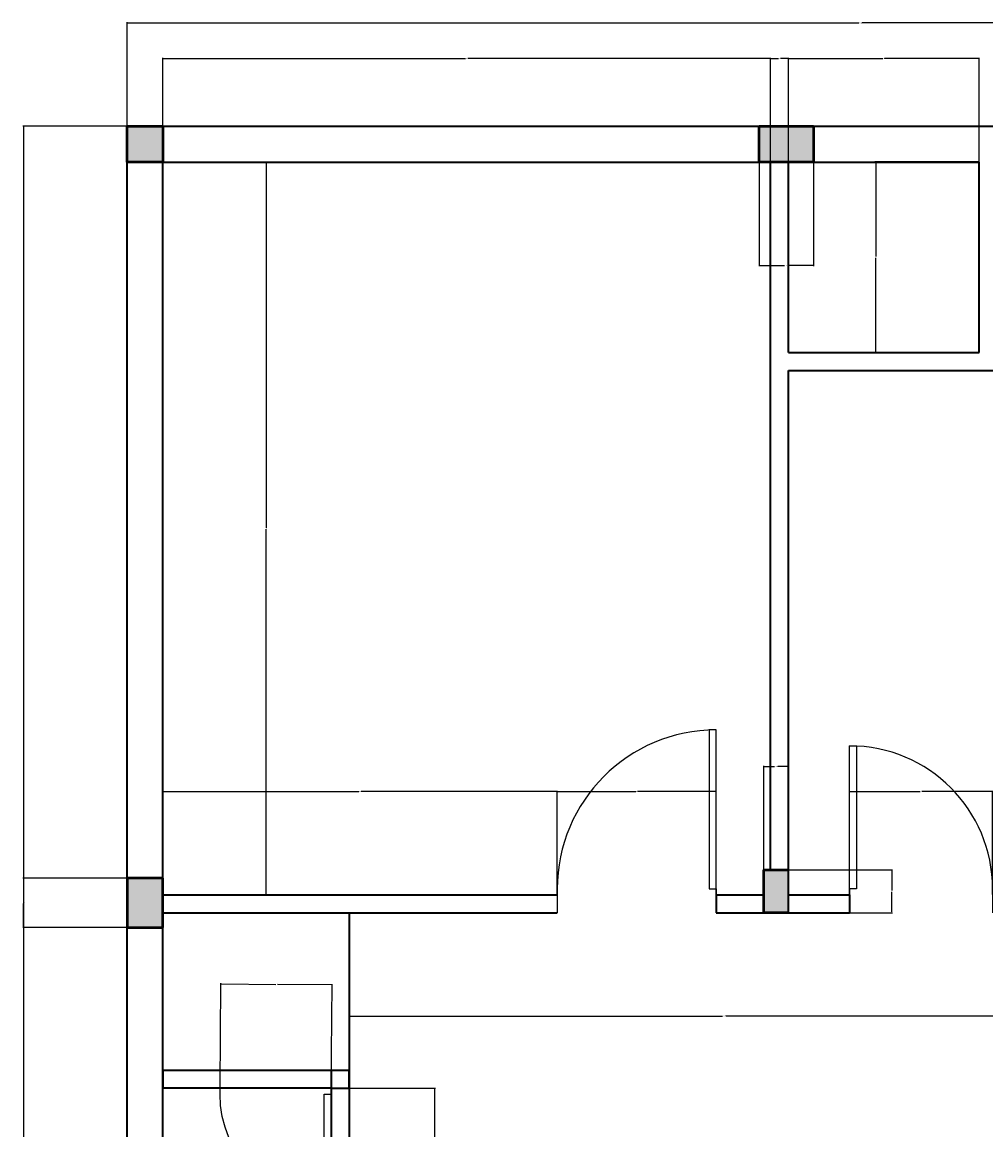
# Model space of a CAD drawing. Units: inches. Extents: x 229 to 651, y 108 to 681.
# Tile 3 of 4: x 229 to 472, y 402 to 681. Entities that reach past the tile are written whole.
import ezdxf

# ---------------------------------------------------------------- set-up
doc = ezdxf.new("R2010")
doc.units = ezdxf.units.IN
doc.header["$MEASUREMENT"] = 0
for name, color, linetype, lineweight in [('A-ANNO-DIMS', 2, 'Continuous', 18), ('A-COLS', 7, 'Continuous', 50), ('A-COLS-PATT', 5, 'Continuous', 13), ('A-DOOR', 3, 'Continuous', 25), ('A-WALL', 7, 'Continuous', 35)]:
    doc.layers.add(name, color=color, linetype=linetype, lineweight=lineweight)
doc.styles.get("Standard").update_dxf_attribs({"font": 'arial.ttf'})
doc.dimstyles.get("Standard").update_dxf_attribs({"dimtxt": 0.18, "dimasz": 0.18, "dimexe": 0.18, "dimexo": 0.0625, "dimgap": 0.09, "dimtad": 0, "dimtih": 1, "dimtoh": 1, "dimdec": 4, "dimzin": 0, "dimdsep": 46, "dimtxsty": 'Standard', "dimcen": 0.09, "dimadec": 0, "dimazin": 0, "dimtfac": 1, "dimtdec": 4, "dimtofl": 0, "dimtmove": 0, "dimatfit": 3, "dimfxl": 1, "dimtolj": 1, "dimtzin": 0, "dimarcsym": 0})

# ---------------------------------------------------------------- blocks, each defined once
blk = doc.blocks.new('*U3')
for p, q in [((0, 0), (0, -6)), ((-40, 0), (-40, -6))]:
    blk.add_line(p, q)
blk.add_lwpolyline([(0, 0), (0, 40), (-1.75, 40), (-1.75, 0)], close=True)
blk.add_arc((0, 0), 40, 90, 180)
blk = doc.blocks.new('*U4')
for p, q in [((0, 0), (0, -6)), ((36, 0), (36, -6))]:
    blk.add_line(p, q)
blk.add_lwpolyline([(0, 0), (0, 36), (1.75, 36), (1.75, 0)], close=True)
blk.add_arc((0, 0), 36, 0, 90)
blk = doc.blocks.new('*U9')
for p, q in [((-28, 0), (-28, -6)), ((0, 0), (0, -6))]:
    blk.add_line(p, q)
blk.add_lwpolyline([(0, 0), (0, 28), (-1.75, 28), (-1.75, 0)], close=True)
blk.add_arc((0, 0), 28, 90, 180)
blk = doc.blocks.new('*D13')
at = {"layer": 'A-ANNO-DIMS', "color": 0, "lineweight": -2, "transparency": 16777216}
for p, q in [((255.74, 655.15), (255.74, 681.3)), ((255.92, 681.12), (439.96, 681.12)), ((624.79, 681.12), (440.75, 681.12)), ((624.97, 655.15), (624.97, 681.3))]:
    blk.add_line(p, q, dxfattribs=at)
at = {"layer": 'A-ANNO-DIMS', "color": 0, "transparency": 16777216}
for points in [[(255.92, 681.15), (255.92, 681.09), (255.74, 681.12)], [(624.79, 681.15), (624.79, 681.09), (624.97, 681.12)]]:
    blk.add_solid(points, dxfattribs=at)
at = {"layer": 'Defpoints', "color": 0, "transparency": 16777216}
for p in [(624.97, 681.12), (255.74, 655.09), (624.97, 655.09)]:
    blk.add_point(p, dxfattribs=at)
at = {"layer": 'A-ANNO-DIMS', "color": 0, "transparency": 16777216, "insert": (440.36, 681.12), "char_height": 0.18, "attachment_point": 5}
blk.add_mtext('\\A1;369.2', dxfattribs=at)
blk = doc.blocks.new('*D14')
at = {"layer": 'A-ANNO-DIMS', "color": 0, "lineweight": -2, "transparency": 16777216}
for p, q in [((255.68, 655.09), (229.53, 655.09)), ((229.71, 654.91), (229.71, 395.02)), ((229.71, 134.77), (229.71, 394.65)), ((255.68, 134.59), (229.53, 134.59))]:
    blk.add_line(p, q, dxfattribs=at)
at = {"layer": 'A-ANNO-DIMS', "color": 0, "transparency": 16777216}
for points in [[(229.68, 654.91), (229.74, 654.91), (229.71, 655.09)], [(229.68, 134.77), (229.74, 134.77), (229.71, 134.59)]]:
    blk.add_solid(points, dxfattribs=at)
at = {"layer": 'Defpoints', "color": 0, "transparency": 16777216}
for p in [(229.71, 655.09), (255.74, 655.09), (255.74, 134.59)]:
    blk.add_point(p, dxfattribs=at)
at = {"layer": 'A-ANNO-DIMS', "color": 0, "transparency": 16777216, "insert": (229.71, 394.84), "char_height": 0.18, "attachment_point": 5}
blk.add_mtext('\\A1;520.5', dxfattribs=at)
blk = doc.blocks.new('*D16')
at = {"layer": 'A-ANNO-DIMS', "color": 0, "lineweight": -2, "transparency": 16777216}
for p, q in [((264.81, 646.09), (290.95, 646.09)), ((290.77, 645.91), (290.77, 554.02)), ((290.77, 461.77), (290.77, 553.65)), ((264.81, 461.59), (290.95, 461.59))]:
    blk.add_line(p, q, dxfattribs=at)
at = {"layer": 'A-ANNO-DIMS', "color": 0, "transparency": 16777216}
for points in [[(290.74, 645.91), (290.8, 645.91), (290.77, 646.09)], [(290.74, 461.77), (290.8, 461.77), (290.77, 461.59)]]:
    blk.add_solid(points, dxfattribs=at)
at = {"layer": 'Defpoints', "color": 0, "transparency": 16777216}
for p in [(264.74, 646.09), (264.74, 461.59), (290.77, 461.59)]:
    blk.add_point(p, dxfattribs=at)
at = {"layer": 'A-ANNO-DIMS', "color": 0, "transparency": 16777216, "insert": (290.77, 553.84), "char_height": 0.18, "attachment_point": 5}
blk.add_mtext('\\A1;184.5', dxfattribs=at)
blk = doc.blocks.new('*D19')
at = {"layer": 'A-ANNO-DIMS', "color": 0, "lineweight": -2, "transparency": 16777216}
for p, q in [((264.74, 646.15), (264.74, 672.3)), ((264.92, 672.12), (340.96, 672.12)), ((417.56, 672.12), (341.52, 672.12)), ((417.74, 646.15), (417.74, 672.3))]:
    blk.add_line(p, q, dxfattribs=at)
at = {"layer": 'A-ANNO-DIMS', "color": 0, "transparency": 16777216}
for points in [[(264.92, 672.15), (264.92, 672.09), (264.74, 672.12)], [(417.56, 672.15), (417.56, 672.09), (417.74, 672.12)]]:
    blk.add_solid(points, dxfattribs=at)
at = {"layer": 'Defpoints', "color": 0, "transparency": 16777216}
for p in [(417.74, 672.12), (264.74, 646.09), (417.74, 646.09)]:
    blk.add_point(p, dxfattribs=at)
at = {"layer": 'A-ANNO-DIMS', "color": 0, "transparency": 16777216, "insert": (341.24, 672.12), "char_height": 0.18, "attachment_point": 5}
blk.add_mtext('\\A1;153', dxfattribs=at)
blk = doc.blocks.new('*D20')
at = {"layer": 'A-ANNO-DIMS', "color": 0, "lineweight": -2, "transparency": 16777216}
for p, q in [((417.74, 646.15), (417.74, 672.3)), ((417.92, 672.12), (419.74, 672.12)), ((422.06, 672.12), (420.25, 672.12)), ((422.24, 646.15), (422.24, 672.3))]:
    blk.add_line(p, q, dxfattribs=at)
at = {"layer": 'A-ANNO-DIMS', "color": 0, "transparency": 16777216}
for points in [[(417.92, 672.15), (417.92, 672.09), (417.74, 672.12)], [(422.06, 672.15), (422.06, 672.09), (422.24, 672.12)]]:
    blk.add_solid(points, dxfattribs=at)
at = {"layer": 'Defpoints', "color": 0, "transparency": 16777216}
for p in [(422.24, 672.12), (417.74, 646.09), (422.24, 646.09)]:
    blk.add_point(p, dxfattribs=at)
at = {"layer": 'A-ANNO-DIMS', "color": 0, "transparency": 16777216, "insert": (419.99, 672.12), "char_height": 0.18, "attachment_point": 5}
blk.add_mtext('\\A1;4.5', dxfattribs=at)
blk = doc.blocks.new('*D21')
at = {"layer": 'A-ANNO-DIMS', "color": 0, "lineweight": -2, "transparency": 16777216}
for p, q in [((422.24, 646.15), (422.24, 672.3)), ((422.42, 672.12), (446.02, 672.12)), ((470.06, 672.12), (446.47, 672.12)), ((470.24, 646.15), (470.24, 672.3))]:
    blk.add_line(p, q, dxfattribs=at)
at = {"layer": 'A-ANNO-DIMS', "color": 0, "transparency": 16777216}
for points in [[(422.42, 672.15), (422.42, 672.09), (422.24, 672.12)], [(470.06, 672.15), (470.06, 672.09), (470.24, 672.12)]]:
    blk.add_solid(points, dxfattribs=at)
at = {"layer": 'Defpoints', "color": 0, "transparency": 16777216}
for p in [(470.24, 672.12), (422.24, 646.09), (470.24, 646.09)]:
    blk.add_point(p, dxfattribs=at)
at = {"layer": 'A-ANNO-DIMS', "color": 0, "transparency": 16777216, "insert": (446.24, 672.12), "char_height": 0.18, "attachment_point": 5}
blk.add_mtext('\\A1;48', dxfattribs=at)
blk = doc.blocks.new('*D24')
at = {"layer": 'A-ANNO-DIMS', "color": 0, "lineweight": -2, "transparency": 16777216}
for p, q in [((470.18, 646.09), (444.03, 646.09)), ((444.21, 645.91), (444.21, 622.27)), ((444.21, 598.27), (444.21, 621.9)), ((470.18, 598.09), (444.03, 598.09))]:
    blk.add_line(p, q, dxfattribs=at)
at = {"layer": 'A-ANNO-DIMS', "color": 0, "transparency": 16777216}
for points in [[(444.18, 645.91), (444.24, 645.91), (444.21, 646.09)], [(444.18, 598.27), (444.24, 598.27), (444.21, 598.09)]]:
    blk.add_solid(points, dxfattribs=at)
at = {"layer": 'Defpoints', "color": 0, "transparency": 16777216}
for p in [(444.21, 646.09), (470.24, 646.09), (470.24, 598.09)]:
    blk.add_point(p, dxfattribs=at)
at = {"layer": 'A-ANNO-DIMS', "color": 0, "transparency": 16777216, "insert": (444.21, 622.09), "char_height": 0.18, "attachment_point": 5}
blk.add_mtext('\\A1;48', dxfattribs=at)
blk = doc.blocks.new('*D30')
at = {"layer": 'A-ANNO-DIMS', "color": 0, "lineweight": -2, "transparency": 16777216}
for p, q in [((264.74, 461.65), (264.74, 487.8)), ((264.92, 487.62), (314.07, 487.62)), ((363.86, 487.62), (314.72, 487.62)), ((364.04, 461.65), (364.04, 487.8))]:
    blk.add_line(p, q, dxfattribs=at)
at = {"layer": 'A-ANNO-DIMS', "color": 0, "transparency": 16777216}
for points in [[(264.92, 487.65), (264.92, 487.59), (264.74, 487.62)], [(363.86, 487.65), (363.86, 487.59), (364.04, 487.62)]]:
    blk.add_solid(points, dxfattribs=at)
at = {"layer": 'Defpoints', "color": 0, "transparency": 16777216}
for p in [(364.04, 487.62), (264.74, 461.59), (364.04, 461.59)]:
    blk.add_point(p, dxfattribs=at)
at = {"layer": 'A-ANNO-DIMS', "color": 0, "transparency": 16777216, "insert": (314.39, 487.62), "char_height": 0.18, "attachment_point": 5}
blk.add_mtext('\\A1;99.3', dxfattribs=at)
blk = doc.blocks.new('*D31')
at = {"layer": 'A-ANNO-DIMS', "color": 0, "lineweight": -2, "transparency": 16777216}
for p, q in [((364.04, 461.65), (364.04, 487.8)), ((364.22, 487.62), (383.82, 487.62)), ((403.86, 487.62), (384.26, 487.62)), ((404.04, 461.65), (404.04, 487.8))]:
    blk.add_line(p, q, dxfattribs=at)
at = {"layer": 'A-ANNO-DIMS', "color": 0, "transparency": 16777216}
for points in [[(364.22, 487.65), (364.22, 487.59), (364.04, 487.62)], [(403.86, 487.65), (403.86, 487.59), (404.04, 487.62)]]:
    blk.add_solid(points, dxfattribs=at)
at = {"layer": 'Defpoints', "color": 0, "transparency": 16777216}
for p in [(404.04, 487.62), (364.04, 461.59), (404.04, 461.59)]:
    blk.add_point(p, dxfattribs=at)
at = {"layer": 'A-ANNO-DIMS', "color": 0, "transparency": 16777216, "insert": (384.04, 487.62), "char_height": 0.18, "attachment_point": 5}
blk.add_mtext('\\A1;40', dxfattribs=at)
blk = doc.blocks.new('*D32')
at = {"layer": 'A-ANNO-DIMS', "color": 0, "lineweight": -2, "transparency": 16777216}
for p, q in [((437.65, 461.65), (437.65, 487.8)), ((437.83, 487.62), (455.43, 487.62)), ((473.47, 487.62), (455.87, 487.62)), ((473.65, 461.65), (473.65, 487.8))]:
    blk.add_line(p, q, dxfattribs=at)
at = {"layer": 'A-ANNO-DIMS', "color": 0, "transparency": 16777216}
for points in [[(437.83, 487.65), (437.83, 487.59), (437.65, 487.62)], [(473.47, 487.65), (473.47, 487.59), (473.65, 487.62)]]:
    blk.add_solid(points, dxfattribs=at)
at = {"layer": 'Defpoints', "color": 0, "transparency": 16777216}
for p in [(473.65, 487.62), (437.65, 461.59), (473.65, 461.59)]:
    blk.add_point(p, dxfattribs=at)
at = {"layer": 'A-ANNO-DIMS', "color": 0, "transparency": 16777216, "insert": (455.65, 487.62), "char_height": 0.18, "attachment_point": 5}
blk.add_mtext('\\A1;36', dxfattribs=at)
blk = doc.blocks.new('*D39')
at = {"layer": 'A-ANNO-DIMS', "color": 0, "lineweight": -2, "transparency": 16777216}
for p, q in [((307.21, 412.88), (333.36, 412.88)), ((333.18, 412.7), (333.18, 375.16)), ((333.18, 337.27), (333.18, 374.8)), ((307.21, 337.09), (333.36, 337.09))]:
    blk.add_line(p, q, dxfattribs=at)
at = {"layer": 'A-ANNO-DIMS', "color": 0, "transparency": 16777216}
for points in [[(333.15, 412.7), (333.21, 412.7), (333.18, 412.88)], [(333.15, 337.27), (333.21, 337.27), (333.18, 337.09)]]:
    blk.add_solid(points, dxfattribs=at)
at = {"layer": 'Defpoints', "color": 0, "transparency": 16777216}
for p in [(307.15, 412.88), (307.15, 337.09), (333.18, 337.09)]:
    blk.add_point(p, dxfattribs=at)
at = {"layer": 'A-ANNO-DIMS', "color": 0, "transparency": 16777216, "insert": (333.18, 374.98), "char_height": 0.18, "attachment_point": 5}
blk.add_mtext('\\A1;75.79', dxfattribs=at)
blk = doc.blocks.new('*D40')
at = {"layer": 'A-ANNO-DIMS', "color": 0, "lineweight": -2, "transparency": 16777216}
for p, q in [((279.15, 413.19), (279.38, 439.34)), ((279.56, 439.16), (293.16, 439.04)), ((307.2, 438.91), (293.6, 439.03)), ((307.15, 412.94), (307.38, 439.09))]:
    blk.add_line(p, q, dxfattribs=at)
at = {"layer": 'A-ANNO-DIMS', "color": 0, "transparency": 16777216}
for points in [[(279.56, 439.19), (279.56, 439.13), (279.38, 439.16)], [(307.2, 438.94), (307.2, 438.88), (307.38, 438.91)]]:
    blk.add_solid(points, dxfattribs=at)
at = {"layer": 'Defpoints', "color": 0, "transparency": 16777216}
for p in [(307.38, 438.91), (279.15, 413.13), (307.15, 412.88)]:
    blk.add_point(p, dxfattribs=at)
at = {"layer": 'A-ANNO-DIMS', "color": 0, "transparency": 16777216, "insert": (293.38, 439.03), "char_height": 0.18, "attachment_point": 5}
blk.add_mtext('\\A1;28', dxfattribs=at)
blk = doc.blocks.new('*D41')
at = {"layer": 'A-ANNO-DIMS', "color": 0, "lineweight": -2, "transparency": 16777216}
for p, q in [((311.65, 457.02), (311.65, 430.88)), ((500.47, 457.02), (500.47, 430.88)), ((311.83, 431.06), (405.61, 431.06)), ((500.29, 431.06), (406.51, 431.06))]:
    blk.add_line(p, q, dxfattribs=at)
at = {"layer": 'A-ANNO-DIMS', "color": 0, "transparency": 16777216}
for points in [[(311.83, 431.09), (311.83, 431.03), (311.65, 431.06)], [(500.29, 431.09), (500.29, 431.03), (500.47, 431.06)]]:
    blk.add_solid(points, dxfattribs=at)
at = {"layer": 'Defpoints', "color": 0, "transparency": 16777216}
for p in [(311.65, 457.09), (500.47, 457.09), (311.65, 431.06)]:
    blk.add_point(p, dxfattribs=at)
at = {"layer": 'A-ANNO-DIMS', "color": 0, "transparency": 16777216, "insert": (406.06, 431.06), "char_height": 0.18, "attachment_point": 5}
blk.add_mtext('\\A1;188.82', dxfattribs=at)
blk = doc.blocks.new('*D73')
at = {"layer": 'A-ANNO-DIMS', "color": 0, "lineweight": -2, "transparency": 16777216}
for p, q in [((414.85, 646.02), (414.85, 619.88)), ((428.54, 646.02), (428.54, 619.88)), ((415.03, 620.06), (421.24, 620.06)), ((428.36, 620.06), (422.15, 620.06))]:
    blk.add_line(p, q, dxfattribs=at)
at = {"layer": 'A-ANNO-DIMS', "color": 0, "transparency": 16777216}
for points in [[(415.03, 620.09), (415.03, 620.03), (414.85, 620.06)], [(428.36, 620.09), (428.36, 620.03), (428.54, 620.06)]]:
    blk.add_solid(points, dxfattribs=at)
at = {"layer": 'Defpoints', "color": 0, "transparency": 16777216}
for p in [(414.85, 646.09), (428.54, 646.09), (414.85, 620.06)]:
    blk.add_point(p, dxfattribs=at)
at = {"layer": 'A-ANNO-DIMS', "color": 0, "transparency": 16777216, "insert": (421.69, 620.06), "char_height": 0.18, "attachment_point": 5}
blk.add_mtext('\\A1;13.684', dxfattribs=at)
blk = doc.blocks.new('*D79')
at = {"layer": 'A-ANNO-DIMS', "color": 0, "lineweight": -2, "transparency": 16777216}
for p, q in [((255.68, 465.8), (229.53, 465.8)), ((229.71, 465.62), (229.71, 459.78)), ((229.71, 453.57), (229.71, 459.41)), ((255.68, 453.39), (229.53, 453.39))]:
    blk.add_line(p, q, dxfattribs=at)
at = {"layer": 'A-ANNO-DIMS', "color": 0, "transparency": 16777216}
for points in [[(229.68, 465.62), (229.74, 465.62), (229.71, 465.8)], [(229.68, 453.57), (229.74, 453.57), (229.71, 453.39)]]:
    blk.add_solid(points, dxfattribs=at)
at = {"layer": 'Defpoints', "color": 0, "transparency": 16777216}
for p in [(229.71, 465.8), (255.74, 465.8), (255.74, 453.39)]:
    blk.add_point(p, dxfattribs=at)
at = {"layer": 'A-ANNO-DIMS', "color": 0, "transparency": 16777216, "insert": (229.71, 459.59), "char_height": 0.18, "attachment_point": 5}
blk.add_mtext('\\A1;12.414', dxfattribs=at)
blk = doc.blocks.new('*D80')
at = {"layer": 'A-ANNO-DIMS', "color": 0, "lineweight": -2, "transparency": 16777216}
for p, q in [((416.07, 467.94), (416.07, 494.08)), ((416.25, 493.9), (418.76, 493.9)), ((422.06, 493.9), (419.55, 493.9)), ((422.24, 467.94), (422.24, 494.08))]:
    blk.add_line(p, q, dxfattribs=at)
at = {"layer": 'A-ANNO-DIMS', "color": 0, "transparency": 16777216}
for points in [[(416.25, 493.93), (416.25, 493.87), (416.07, 493.9)], [(422.06, 493.93), (422.06, 493.87), (422.24, 493.9)]]:
    blk.add_solid(points, dxfattribs=at)
at = {"layer": 'Defpoints', "color": 0, "transparency": 16777216}
for p in [(422.24, 493.9), (416.07, 467.87), (422.24, 467.87)]:
    blk.add_point(p, dxfattribs=at)
at = {"layer": 'A-ANNO-DIMS', "color": 0, "transparency": 16777216, "insert": (419.16, 493.9), "char_height": 0.18, "attachment_point": 5}
blk.add_mtext('\\A1;6.172', dxfattribs=at)
blk = doc.blocks.new('*D81')
at = {"layer": 'A-ANNO-DIMS', "color": 0, "lineweight": -2, "transparency": 16777216}
for p, q in [((422.31, 467.87), (448.45, 467.87)), ((448.27, 467.69), (448.27, 462.66)), ((448.27, 457.27), (448.27, 462.3)), ((422.31, 457.09), (448.45, 457.09))]:
    blk.add_line(p, q, dxfattribs=at)
at = {"layer": 'A-ANNO-DIMS', "color": 0, "transparency": 16777216}
for points in [[(448.24, 467.69), (448.3, 467.69), (448.27, 467.87)], [(448.24, 457.27), (448.3, 457.27), (448.27, 457.09)]]:
    blk.add_solid(points, dxfattribs=at)
at = {"layer": 'Defpoints', "color": 0, "transparency": 16777216}
for p in [(422.24, 467.87), (422.24, 457.09), (448.27, 457.09)]:
    blk.add_point(p, dxfattribs=at)
at = {"layer": 'A-ANNO-DIMS', "color": 0, "transparency": 16777216, "insert": (448.27, 462.48), "char_height": 0.18, "attachment_point": 5}
blk.add_mtext('\\A1;10.787', dxfattribs=at)

msp = doc.modelspace()

# ---------------------------------------------------------------- hatches: boundary and pattern name
at = {"layer": 'A-COLS-PATT'}
h = msp.add_hatch(color=256, dxfattribs=at)
h.dxf.hatch_style = 1
h.paths.add_polyline_path([(264.7698, 655.0869), (255.744, 655.0869), (255.744, 646.0869), (264.7698, 646.0869)])
h.paths.add_polyline_path([(428.5355, 655.0869), (414.8518, 655.0869), (414.8518, 646.0869), (428.5355, 646.0869)])
h.paths.add_polyline_path([(579.744, 655.0869), (568.5366, 655.0869), (568.5366, 646.0869), (570.744, 646.0869), (579.744, 646.0869)])
h.paths.add_polyline_path([(579.744, 468.8158), (570.744, 468.8158), (570.744, 457.0869), (579.744, 457.0869)])
h.paths.add_polyline_path([(422.244, 467.874), (416.0718, 467.874), (416.0718, 457.0869), (422.244, 457.0869)])
h.paths.add_polyline_path([(264.744, 465.8018), (255.744, 465.8018), (255.744, 453.3882), (264.744, 453.3882), (264.744, 457.0869)])
h.paths.add_polyline_path([(264.744, 337.0869), (255.744, 337.0869), (255.744, 328.0161), (264.744, 328.0161)])
h.paths.add_polyline_path([(425.426, 337.0869), (411.84, 337.0869), (411.84, 328.0869), (425.426, 328.0869)])
h.paths.add_polyline_path([(579.744, 337.0869), (570.744, 337.0869), (570.744, 328.0869), (579.744, 328.0869)])
h.paths.add_polyline_path([(579.744, 188.4262), (570.744, 188.4262), (570.744, 178.0508), (579.744, 178.0508)])
h.paths.add_polyline_path([(413.7248, 169.0053), (405.843, 169.0053), (405.843, 162.8404), (413.7248, 162.8404)])
h.paths.add_polyline_path([(264.744, 180.6917), (255.744, 180.6917), (255.744, 171.3369), (264.744, 171.3369)])

# ---------------------------------------------------------------- linework, layer by layer
at = {"layer": 'A-COLS'}
for p, q in [((255.744, 646.0869), (255.744, 655.0869)), ((255.744, 655.0869), (264.7698, 655.0869)), ((264.7698, 655.0869), (264.7698, 646.0869)), ((414.8518, 646.0869), (414.8518, 655.0869)), ((414.8518, 655.0869), (428.5355, 655.0869)), ((428.5355, 655.0869), (428.5355, 646.0869)), ((264.744, 646.0869), (255.744, 646.0869)), ((428.5355, 646.0869), (414.8518, 646.0869)), ((264.744, 465.8018), (255.744, 465.8018)), ((255.744, 465.8018), (255.744, 453.3882)), ((264.744, 457.0869), (264.744, 465.8018)), ((416.0718, 457.0869), (416.0718, 467.874)), ((416.0718, 467.874), (422.244, 467.874)), ((264.744, 453.3882), (264.744, 457.0869)), ((422.244, 457.0869), (416.0718, 457.0869)), ((255.744, 453.3882), (264.744, 453.3882))]:
    msp.add_line(p, q, dxfattribs=at)
at = {"layer": 'A-WALL'}
for p, q in [((255.744, 655.0869), (579.744, 655.0869)), ((255.744, 139.0869), (255.744, 655.0869)), ((264.744, 646.0869), (417.744, 646.0869)), ((264.744, 461.5869), (264.744, 646.0869)), ((417.744, 646.0869), (414.8518, 646.0869)), ((417.744, 467.874), (417.744, 646.0869)), ((422.244, 646.0869), (470.244, 646.0869)), ((422.244, 598.0869), (422.244, 646.0869)), ((470.244, 598.0869), (470.244, 646.0869)), ((422.244, 598.0869), (470.244, 598.0869)), ((422.244, 457.0869), (422.244, 593.5869)), ((422.244, 593.5869), (474.744, 593.5869)), ((264.744, 461.5869), (364.0385, 461.5869)), ((404.0385, 461.5869), (404.0385, 457.0869)), ((404.0385, 461.5869), (416.0718, 461.5869)), ((422.244, 461.5869), (437.6462, 461.5869)), ((437.6462, 461.5869), (437.6462, 457.0869)), ((264.744, 457.0869), (311.6505, 457.0869)), ((264.744, 337.0869), (264.744, 457.0869)), ((311.6505, 457.0869), (311.6505, 337.0869)), ((311.6505, 457.0869), (364.0385, 457.0869)), ((404.0385, 457.0869), (422.244, 457.0869)), ((422.244, 457.0869), (437.6462, 457.0869)), ((311.6505, 417.3792), (264.744, 417.3792)), ((264.744, 417.3792), (264.744, 412.8792)), ((307.1505, 417.1791), (307.1505, 337.0869)), ((311.6505, 412.8792), (311.6505, 417.3792)), ((307.1505, 412.8792), (264.744, 412.8792)), ((307.1505, 412.8792), (311.6505, 412.8792))]:
    msp.add_line(p, q, dxfattribs=at)

# ---------------------------------------------------------------- block references
at = {"layer": 'A-DOOR'}
for name, p in [('*U3', (404.0385, 463.0869)), ('*U4', (437.6462, 463.0869))]:
    msp.add_blockref(name, p, dxfattribs=at)
at = {"layer": 'A-DOOR', "xscale": -1, "rotation": 180}
msp.add_blockref('*U9', (307.1505, 411.3792), dxfattribs=at)

# ---------------------------------------------------------------- dimensions: what is measured, and where the dimension line sits
at = {"layer": 'A-ANNO-DIMS'}
for base, p1, p2, override, picture, middle in [((624.9705, 681.1169), (255.744, 655.0869), (624.9705, 655.0869), {"dimdec": 1, "dimlfac": 1, "dimrnd": 0, "dimzin": 0, "dimdsep": 46, "dimlunit": 2}, '*D13', (440.3573, 681.1169)), ((417.744, 672.1169), (264.744, 646.0869), (417.744, 646.0869), {"dimdec": 0, "dimlfac": 1, "dimrnd": 0, "dimzin": 0, "dimdsep": 46, "dimlunit": 2}, '*D19', (341.244, 672.1169)), ((422.244, 672.1169), (417.744, 646.0869), (422.244, 646.0869), {"dimdec": 1, "dimlfac": 1, "dimrnd": 0, "dimzin": 0, "dimdsep": 46, "dimlunit": 2}, '*D20', (419.994, 672.1169)), ((470.244, 672.1169), (422.244, 646.0869), (470.244, 646.0869), {"dimdec": 0, "dimlfac": 1, "dimrnd": 0, "dimzin": 0, "dimdsep": 46, "dimlunit": 2}, '*D21', (446.244, 672.1169)), ((422.244, 493.904), (416.0718, 467.874), (422.244, 467.874), {"dimdec": 3, "dimlfac": 1, "dimrnd": 0, "dimzin": 0, "dimdsep": 46, "dimlunit": 2}, '*D80', (419.1579, 493.904)), ((364.0385, 487.6169), (264.744, 461.5869), (364.0385, 461.5869), {"dimdec": 1, "dimlfac": 1, "dimrnd": 0, "dimzin": 0, "dimdsep": 46, "dimlunit": 2}, '*D30', (314.3913, 487.6169)), ((404.0385, 487.6169), (364.0385, 461.5869), (404.0385, 461.5869), {"dimdec": 0, "dimlfac": 1, "dimrnd": 0, "dimzin": 0, "dimdsep": 46, "dimlunit": 2}, '*D31', (384.0385, 487.6169)), ((473.6462, 487.6169), (437.6462, 461.5869), (473.6462, 461.5869), {"dimdec": 0, "dimlfac": 1, "dimrnd": 0, "dimzin": 0, "dimdsep": 46, "dimlunit": 2}, '*D32', (455.6462, 487.6169))]:
    dim = msp.add_linear_dim(base=base, p1=p1, p2=p2, dimstyle='Standard', override=override, dxfattribs=at)
    dim.commit()
    dim.dimension.update_dxf_attribs({"geometry": picture, "text_midpoint": middle})
for base, p1, p2, angle, override, picture, middle in [((229.714, 655.0869), (255.744, 134.5869), (255.744, 655.0869), 90, {"dimdec": 1, "dimlfac": 1, "dimrnd": 0, "dimzin": 0, "dimdsep": 46, "dimlunit": 2}, '*D14', (229.714, 394.8369)), ((290.774, 461.5869), (264.744, 646.0869), (264.744, 461.5869), 270, {"dimdec": 1, "dimlfac": 1, "dimrnd": 0, "dimzin": 0, "dimdsep": 46, "dimlunit": 2}, '*D16', (290.774, 553.8369)), ((414.8518, 620.0569), (428.5355, 646.0869), (414.8518, 646.0869), 180, {"dimdec": 3, "dimlfac": 1, "dimrnd": 0, "dimzin": 0, "dimdsep": 46, "dimlunit": 2}, '*D73', (421.6936, 620.0569)), ((444.214, 646.0869), (470.244, 598.0869), (470.244, 646.0869), 90, {"dimdec": 0, "dimlfac": 1, "dimrnd": 0, "dimzin": 0, "dimdsep": 46, "dimlunit": 2}, '*D24', (444.214, 622.0869)), ((229.714, 465.8018), (255.744, 453.3882), (255.744, 465.8018), 90, {"dimdec": 3, "dimlfac": 1, "dimrnd": 0, "dimzin": 0, "dimdsep": 46, "dimlunit": 2}, '*D79', (229.714, 459.595)), ((448.274, 457.0869), (422.244, 467.874), (422.244, 457.0869), 270, {"dimdec": 3, "dimlfac": 1, "dimrnd": 0, "dimzin": 0, "dimdsep": 46, "dimlunit": 2}, '*D81', (448.274, 462.4804)), ((311.6505, 431.0569), (500.4705, 457.0869), (311.6505, 457.0869), 180, {"dimdec": 2, "dimlfac": 1, "dimrnd": 0, "dimzin": 0, "dimdsep": 46, "dimlunit": 2}, '*D41', (406.0605, 431.0569)), ((307.3829, 438.9082), (279.1505, 413.1292), (307.1505, 412.8792), 359.488444, {"dimdec": 0, "dimlfac": 1, "dimrnd": 0, "dimzin": 0, "dimdsep": 46, "dimlunit": 2}, '*D40', (293.3829, 439.0332)), ((333.1805, 337.0869), (307.1505, 412.8792), (307.1505, 337.0869), 270, {"dimdec": 2, "dimlfac": 1, "dimrnd": 0, "dimzin": 0, "dimdsep": 46, "dimlunit": 2}, '*D39', (333.1805, 374.983))]:
    dim = msp.add_linear_dim(base=base, p1=p1, p2=p2, angle=angle, dimstyle='Standard', override=override, dxfattribs=at)
    dim.commit()
    dim.dimension.update_dxf_attribs({"geometry": picture, "text_midpoint": middle})

doc.saveas('drawing.dxf')
